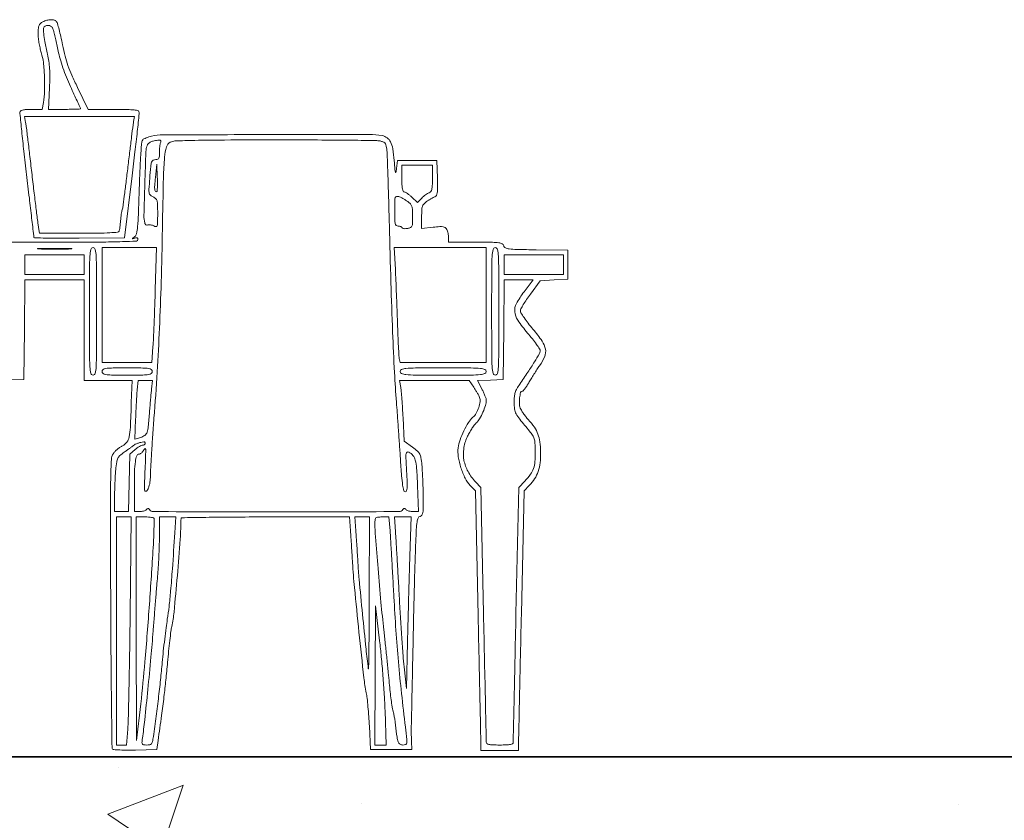
# Model space of a CAD drawing. Units: inches. Extents: x 2416 to 3391, y 1375 to 2496.
# Tile 8 of 13: x 3014 to 3044, y 2142 to 2166. Entities that reach past the tile are written whole.
import ezdxf

# ---------------------------------------------------------------- set-up
doc = ezdxf.new("R2010")
doc.units = ezdxf.units.IN
for name, color, linetype, lineweight in [('A-FLOR-PATT', 252, 'Continuous', 13), ('A-FURN', 8, 'Continuous', 18), ('A-SECT', 7, 'Continuous', 35)]:
    doc.layers.add(name, color=color, linetype=linetype, lineweight=lineweight)

msp = doc.modelspace()

# ---------------------------------------------------------------- hatches: boundary and pattern name
at = {"layer": 'A-FLOR-PATT'}
h = msp.add_hatch(dxfattribs=at)
h.set_pattern_fill('AR-CONC', color=256, scale=0.13, style=0)
h.paths.add_polyline_path([(2904.1924, 2125.8608), (3202.6924, 2125.8608), (3202.6924, 2143.8608), (2904.1924, 2143.8608)])

# ---------------------------------------------------------------- linework, layer by layer
at = {"layer": 'A-FURN'}
for points in [[(3014.6302, 2166.3653, 0.062101), (3014.5576, 2166.3165, 0.115801), (3014.5165, 2166.2593, 0.077294), (3014.4957, 2166.174, 0.016831), (3014.488, 2166.0225, 0.029474), (3014.4933, 2165.8947, 0.01481), (3014.5143, 2165.7345, 0.014652), (3014.5459, 2165.5696, 0.021013), (3014.5842, 2165.4259, -0.046916), (3014.6482, 2165.1238, -0.018058), (3014.6821, 2164.696, -0.01826), (3014.6849, 2164.2529, -0.033407), (3014.6499, 2163.8934), (3014.6158, 2163.6872), (3014.2913, 2163.6872, 0.014838), (3014.1492, 2163.683, 0.034143), (3014.0431, 2163.6694, 0.045195), (3013.9703, 2163.6479, 0.209973), (3013.9401, 2163.6175, 0.116556), (3013.9326, 2163.5615, 0.000649), (3013.9862, 2163.0221, 0.002747), (3014.0516, 2162.4062, 0.001736), (3014.1343, 2161.6884, -0.000302), (3014.219, 2160.9718, -0.000484), (3014.2903, 2160.36, -0.00008), (3014.3529, 2159.8181, -0.028704), (3014.3552, 2159.7776, 0.404392), (3014.3769, 2159.7552, 0.001815), (3014.7367, 2159.7444, 0.00627), (3015.1761, 2159.7383, 0.002975), (3015.7423, 2159.741), (3017.1294, 2159.7557), (3017.366, 2161.6502, 0.001761), (3017.4547, 2162.3815, 0.002787), (3017.5251, 2163.0091, 0.00066), (3017.5828, 2163.5587, 0.117999), (3017.5753, 2163.616, 0.260793), (3017.5322, 2163.6518, 0.023463), (3017.388, 2163.6717, 0.018121), (3017.1613, 2163.6839, 0.00441), (3016.7867, 2163.6872), (3016.0255, 2163.6872), (3015.6938, 2164.3608, -0.009259), (3015.5181, 2164.735, -0.020813), (3015.4021, 2165.0264, -0.022433), (3015.3159, 2165.3126, -0.012613), (3015.2358, 2165.6667, 0.005681), (3015.1835, 2165.914, 0.007954), (3015.1308, 2166.1335, 0.00512), (3015.0819, 2166.3158, 0.098688), (3015.0556, 2166.3678, 0.147434), (3014.9862, 2166.4165, 0.081537), (3014.8831, 2166.4329, 0.066769), (3014.7594, 2166.4155, 0.049048)], [(3014.9677, 2166.0788, -0.002772), (3014.9895, 2165.9854, -0.000537), (3015.0278, 2165.8163, -0.000571), (3015.072, 2165.619, -0.000528), (3015.117, 2165.4164, 0.019587), (3015.1803, 2165.1751, 0.01148), (3015.274, 2164.8914, 0.011132), (3015.386, 2164.5972, 0.012912), (3015.5059, 2164.3227, -0.001196), (3015.6129, 2164.0929, -0.001914), (3015.703, 2163.8961, -0.000347), (3015.7817, 2163.722, -0.1064), (3015.7849, 2163.707, -0.400461), (3015.7772, 2163.699, -0.00162), (3015.6418, 2163.693, -0.006359), (3015.4846, 2163.6886, -0.003817), (3015.2979, 2163.6872), (3014.8109, 2163.6872), (3014.8378, 2164.3414, 0.008389), (3014.8458, 2164.6704, 0.016295), (3014.8393, 2164.9332, 0.019582), (3014.8174, 2165.1589, 0.022353), (3014.7784, 2165.3724, -0.007236), (3014.6949, 2165.7627, -0.026165), (3014.6584, 2166.0142, -0.038745), (3014.6561, 2166.1759, -0.286498), (3014.699, 2166.2358, -0.083407), (3014.7937, 2166.2575, -0.147957), (3014.8708, 2166.239, -0.136318), (3014.929, 2166.1791, -0.066322)], [(3017.4133, 2163.316, 0.016785), (3017.3961, 2163.2107, 0.000753), (3017.3495, 2162.8458, 0.001264), (3017.296, 2162.4126, 0.000904), (3017.2383, 2161.9276, -0.001537), (3017.1805, 2161.4475, -0.002318), (3017.1269, 2161.0296, -0.000902), (3017.0786, 2160.6711, -0.054242), (3017.0629, 2160.608, 0.04182), (3017.0499, 2160.561, 0.008846), (3017.0357, 2160.477, 0.009204), (3017.0227, 2160.3788, 0.00862), (3017.013, 2160.278, -0.007229), (3017.0037, 2160.1783, -0.008244), (3016.9918, 2160.0831, -0.007575), (3016.9792, 2160.0028, -0.045269), (3016.9683, 2159.9619, -0.287901), (3016.9218, 2159.9259, -0.010483), (3016.6886, 2159.908, -0.011347), (3016.3351, 2159.8962, -0.002603), (3015.7378, 2159.8931), (3014.5324, 2159.8931), (3014.5, 2160.0718, -0.01368), (3014.481, 2160.1958, -0.000634), (3014.4284, 2160.618, -0.001051), (3014.3678, 2161.1195, -0.000754), (3014.3021, 2161.6802, 0.000637), (3014.2364, 2162.2409, 0.000888), (3014.1762, 2162.7424, 0.000535), (3014.1242, 2163.1647, 0.011573), (3014.106, 2163.2886), (3014.0753, 2163.4673), (3015.7593, 2163.4673), (3017.4432, 2163.4673)], [(3024.9595, 2162.7183, -0.041596), (3025.0477, 2162.6929, -0.109367), (3025.1024, 2162.657, -0.109052), (3025.1368, 2162.6013, -0.041219), (3025.16, 2162.5121, -0.033548), (3025.1735, 2162.3846, -0.000693), (3025.1969, 2161.7445, -0.00162), (3025.2208, 2160.9959, -0.001089), (3025.2435, 2160.1406, 0.001508), (3025.2916, 2158.3818, 0.00236), (3025.3448, 2156.869, 0.002712), (3025.4011, 2155.6246, 0.006937), (3025.4593, 2154.7244, -0.001348), (3025.4847, 2154.389, -0.000561), (3025.5174, 2153.9361, -0.000555), (3025.5512, 2153.4511, -0.000719), (3025.5811, 2153.0061, 0.002808), (3025.62, 2152.4624, 0.016404), (3025.6514, 2152.1773, 0.024859), (3025.6838, 2152.0105, 0.345), (3025.7291, 2151.9751, 0.316573), (3025.7694, 2152.0034, 0.06895), (3025.7879, 2152.0914, 0.02766), (3025.7902, 2152.2605, 0.003877), (3025.773, 2152.6095, -0.002437), (3025.752, 2153.011, -0.039677), (3025.7563, 2153.1458, -0.244576), (3025.7858, 2153.1897, -0.253054), (3025.8378, 2153.1899, -0.098246), (3025.9659, 2153.0848, -0.107804), (3026.039, 2152.942, -0.048185), (3026.0788, 2152.6983, -0.006257), (3026.1067, 2152.1715), (3026.1392, 2151.3702), (3025.9768, 2151.3702, -0.033091), (3025.9103, 2151.3746, -0.032649), (3025.8446, 2151.3878, -0.034456), (3025.7888, 2151.407, -0.096488), (3025.7547, 2151.43, 0.047458), (3025.7247, 2151.4547, 0.150038), (3025.7001, 2151.4623, 0.181024), (3025.6785, 2151.4542, 0.075363), (3025.6579, 2151.43, -0.259763), (3025.5466, 2151.3678, -0.00016), (3021.7784, 2151.3666, -0.00016), (3018.0103, 2151.3678, -0.259763), (3017.8989, 2151.43, 0.075363), (3017.8784, 2151.4542, 0.181024), (3017.8567, 2151.4623, 0.150038), (3017.8321, 2151.4547, 0.047458), (3017.8022, 2151.43, -0.093185), (3017.7686, 2151.407, -0.03527), (3017.7147, 2151.3878, -0.033428), (3017.6518, 2151.3746, -0.034775), (3017.5885, 2151.3702), (3017.4345, 2151.3702), (3017.4345, 2152.0782, -0.006222), (3017.4409, 2152.5964, -0.027247), (3017.4652, 2152.9016, -0.047529), (3017.5067, 2153.0799, -0.32225), (3017.5761, 2153.1298, 0.107986), (3017.6079, 2153.1367, 0.054516), (3017.6433, 2153.1579, 0.050469), (3017.6767, 2153.1889, 0.052739), (3017.7026, 2153.2256, -0.02608), (3017.7245, 2153.2604, -0.050192), (3017.7461, 2153.2853, -0.081722), (3017.7641, 2153.2973, -0.359139), (3017.7755, 2153.2943, -0.15971), (3017.7827, 2153.2713, -0.001591), (3017.78, 2153.0975, -0.004999), (3017.7742, 2152.8962, -0.003197), (3017.7637, 2152.6624, 0.004132), (3017.7535, 2152.427, 0.006129), (3017.7488, 2152.2207, 0.002969), (3017.748, 2152.0458, 0.11422), (3017.7569, 2152.008, 0.508205), (3017.8077, 2151.999, 0.112529), (3017.8653, 2152.087, 0.050052), (3017.9125, 2152.2672, 0.040546), (3017.9276, 2152.4667, -0.015334), (3017.9323, 2152.6585, -0.001578), (3017.9588, 2153.1106, -0.001966), (3017.9943, 2153.6492, -0.001569), (3018.0366, 2154.2295, 0.003613), (3018.1341, 2155.6473, 0.004281), (3018.2051, 2156.9884, 0.00402), (3018.2563, 2158.3988, 0.002606), (3018.2939, 2160.0306, -0.001427), (3018.3264, 2161.6066, -0.016729), (3018.3614, 2162.22, -0.044224), (3018.4194, 2162.5408, -0.211984), (3018.5342, 2162.6813, -0.108467), (3018.6792, 2162.7187, -0.003462), (3019.2892, 2162.7363, -0.004434), (3020.1924, 2162.7481, -0.000997), (3021.7303, 2162.7516, -0.001043), (3022.9149, 2162.7495, -0.001602), (3023.9406, 2162.7422, -0.000518), (3024.8287, 2162.7321, -0.046286)], [(3018.2377, 2162.6655, 0.050508), (3018.2248, 2162.618, 0.013659), (3018.2141, 2162.5407, 0.013682), (3018.2068, 2162.4519, 0.013799), (3018.2043, 2162.363, -0.018316), (3018.2001, 2162.2491, -0.096973), (3018.1837, 2162.1891, -0.179316), (3018.1513, 2162.1585, -0.100622), (3018.0976, 2162.1476, 0.12004), (3018.0115, 2162.1266, 0.195826), (3017.9634, 2162.0702, 0.057245), (3017.9368, 2161.9425, 0.003765), (3017.9055, 2161.5668, 0.004039), (3017.8833, 2161.238, 0.060235), (3017.8902, 2161.1233, 0.16542), (3017.9266, 2161.0582, 0.076736), (3018.0085, 2161.0044, -0.076881), (3018.0886, 2160.9518, -0.142342), (3018.1292, 2160.8861, -0.061734), (3018.146, 2160.7732, -0.00604), (3018.1493, 2160.4972, -0.003502), (3018.1473, 2160.2093, -0.069301), (3018.1339, 2160.1221, -0.344095), (3018.0994, 2160.0977, -0.111915), (3018.035, 2160.1154, 0.041765), (3017.9858, 2160.1367, 0.038588), (3017.9324, 2160.1501, 0.040889), (3017.8828, 2160.1545, 0.093547), (3017.846, 2160.1479, -0.120448), (3017.8157, 2160.144, -0.121496), (3017.7871, 2160.1546, -0.108755), (3017.7645, 2160.1785, -0.081976), (3017.7511, 2160.2124, -0.059517), (3017.7298, 2160.4363, -0.001663), (3017.7566, 2161.4086, -0.001289), (3017.7896, 2162.3985, -0.080665), (3017.8238, 2162.5695, -0.101839), (3017.8673, 2162.6388, -0.091995), (3017.9361, 2162.6883, -0.062829), (3018.0405, 2162.7223, -0.02224), (3018.1964, 2162.7449, -0.10297), (3018.225, 2162.7419, -0.197977), (3018.2423, 2162.7273, -0.154104), (3018.2468, 2162.7014, -0.058414)], [(3018.1244, 2161.1695, -0.395847), (3018.0853, 2161.1683, -0.188529), (3018.0602, 2161.217, -0.04324), (3018.0579, 2161.3556, -0.008525), (3018.0795, 2161.6034), (3018.1218, 2162.0101), (3018.1381, 2161.6048, -0.007181), (3018.1422, 2161.4474, -0.010754), (3018.1408, 2161.3098, -0.005966), (3018.1358, 2161.1951, -0.184544)], [(3026.5623, 2161.5739, -0.007704), (3026.5588, 2161.3473, -0.048789), (3026.544, 2161.233, -0.111409), (3026.5134, 2161.1693, -0.14956), (3026.461, 2161.1331, 0.058669), (3026.4134, 2161.1116, 0.022268), (3026.3527, 2161.0713, 0.021691), (3026.2899, 2161.0211, 0.024771), (3026.2345, 2160.9677), (3026.1094, 2160.8345), (3025.9372, 2160.9959, 0.018241), (3025.8662, 2161.0577, 0.022282), (3025.7953, 2161.11, 0.021517), (3025.733, 2161.148, 0.125972), (3025.6962, 2161.1576, -0.306893), (3025.6642, 2161.1794, -0.052792), (3025.6435, 2161.254, -0.032091), (3025.631, 2161.3776, -0.009182), (3025.6275, 2161.5702), (3025.6275, 2161.9826), (3026.0949, 2161.9826), (3026.5623, 2161.9826)], [(3025.8051, 2160.8648, -0.04726), (3025.8894, 2160.7893, -0.105675), (3025.933, 2160.7156, -0.06907), (3025.9526, 2160.6116, -0.012071), (3025.9574, 2160.4116, -0.007911), (3025.954, 2160.1971, -0.089309), (3025.9364, 2160.1142, -0.189388), (3025.8942, 2160.07, -0.06065), (3025.8062, 2160.0415, -0.032494), (3025.7469, 2160.034, -0.04645), (3025.694, 2160.0356, -0.05614), (3025.6541, 2160.0452, -0.222131), (3025.6367, 2160.0626, 0.149945), (3025.6221, 2160.082, 0.060016), (3025.5927, 2160.0983, 0.052195), (3025.5546, 2160.1093, 0.044695), (3025.5129, 2160.1131, -0.18104), (3025.4566, 2160.1342, -0.159918), (3025.4244, 2160.1883, -0.050048), (3025.4103, 2160.3044, -0.005016), (3025.4075, 2160.5842, -0.003519), (3025.4097, 2160.8921, -0.065713), (3025.4237, 2160.9879, -0.288466), (3025.4606, 2161.0211, -0.120126), (3025.5302, 2161.0163, -0.034306), (3025.5879, 2160.9935, -0.014795), (3025.6616, 2160.9558, -0.014559), (3025.7378, 2160.9108, -0.018684)], [(3015.4714, 2159.4124, -0.006561), (3015.2639, 2159.4066, -0.003649), (3015.0108, 2159.4047, -0.003639), (3014.7546, 2159.4066, -0.005878), (3014.5366, 2159.4123, -0.030672), (3014.4692, 2159.419, -0.903981), (3014.4695, 2159.4253, -0.008594), (3014.6526, 2159.4296, -0.001615), (3014.9876, 2159.4307, -0.001661), (3015.3231, 2159.4297, -0.007856), (3015.5153, 2159.4254, -0.862966), (3015.516, 2159.419, -0.053751)], [(3016.2798, 2157.5012, -0.000789), (3016.2778, 2156.2278, -0.013281), (3016.2653, 2155.8069, -0.040964), (3016.2369, 2155.6029, -0.351139), (3016.1698, 2155.5492, -0.351139), (3016.1027, 2155.6029, -0.040964), (3016.0743, 2155.8069, -0.013281), (3016.0618, 2156.2278, -0.000789), (3016.0598, 2157.5012, -0.000789), (3016.0618, 2158.7746, -0.013281), (3016.0743, 2159.1955, -0.040964), (3016.1027, 2159.3995, -0.351139), (3016.1698, 2159.4532, -0.351139), (3016.2369, 2159.3995, -0.040964), (3016.2653, 2159.1955, -0.013281), (3016.2778, 2158.7746, -0.000789)], [(3018.0752, 2158.1748, -0.001517), (3018.0589, 2157.6501, -0.001562), (3018.0395, 2157.1306, -0.001509), (3018.0199, 2156.6803, -0.006657), (3018.0041, 2156.4152), (3017.9689, 2155.9341), (3017.2068, 2155.9341), (3016.4447, 2155.9341), (3016.4447, 2157.6937), (3016.4447, 2159.4532), (3017.2779, 2159.4532), (3018.1111, 2159.4532)], [(3028.2119, 2157.6937), (3028.2119, 2155.9341), (3026.8932, 2155.9341), (3025.5746, 2155.9341), (3025.5495, 2156.0578, -0.035598), (3025.5384, 2156.1435, -0.001758), (3025.5229, 2156.4279, -0.002835), (3025.5076, 2156.7662, -0.002044), (3025.4942, 2157.1438, 0.001348), (3025.4799, 2157.5615, 0.001011), (3025.4621, 2158.0213, 0.001022), (3025.4435, 2158.4539, 0.002346), (3025.4274, 2158.7797), (3025.3908, 2159.4532), (3026.8013, 2159.4532), (3028.2119, 2159.4532)], [(3028.5968, 2157.5012, -0.000789), (3028.5948, 2156.2278, -0.013281), (3028.5822, 2155.8069, -0.040964), (3028.5539, 2155.6029, -0.351139), (3028.4868, 2155.5492, -0.351139), (3028.4197, 2155.6029, -0.040964), (3028.3913, 2155.8069, -0.013281), (3028.3788, 2156.2278, -0.000789), (3028.3768, 2157.5012, -0.000789), (3028.3788, 2158.7746, -0.013281), (3028.3913, 2159.1955, -0.040964), (3028.4197, 2159.3995, -0.351139), (3028.4868, 2159.4532, -0.351139), (3028.5539, 2159.3995, -0.040964), (3028.5822, 2159.1955, -0.013281), (3028.5948, 2158.7746, -0.000789)], [(3029.3684, 2158.0979, 0.036037), (3029.1362, 2157.7403, 0.148447), (3029.0832, 2157.4906, 0.129492), (3029.1748, 2157.2343, 0.024803), (3029.4765, 2156.8376, -0.008208), (3029.624, 2156.6566, -0.011718), (3029.7484, 2156.4908, -0.007772), (3029.8461, 2156.3494, -0.148348), (3029.8615, 2156.2987, -0.130297), (3029.8376, 2156.2086, -0.007082), (3029.6871, 2155.9532, -0.010099), (3029.4883, 2155.6408, -0.005901), (3029.2382, 2155.2743, 0.023411), (3029.1482, 2155.132, 0.053399), (3029.0976, 2155.0156, 0.052936), (3029.0725, 2154.8906, 0.022659), (3029.0646, 2154.7201, 0.034382), (3029.0789, 2154.5083, 0.08877), (3029.1259, 2154.3631, 0.048451), (3029.2357, 2154.1981, 0.004972), (3029.5356, 2153.8375, -0.031451), (3029.6314, 2153.7091, -0.076691), (3029.6799, 2153.6019, -0.05417), (3029.7027, 2153.464, -0.009879), (3029.7119, 2153.2051, -0.021459), (3029.7034, 2152.8923, -0.068458), (3029.6606, 2152.6883, -0.075136), (3029.5668, 2152.5138, -0.029552), (3029.39, 2152.305), (3029.2066, 2152.1125), (3029.1216, 2148.2468, 0.000042), (3029.089, 2146.7591, 0.000068), (3029.0616, 2145.4933, 0.000009), (3029.0373, 2144.3653, 0.005374), (3029.0367, 2144.3015, -0.262499), (3029.0147, 2144.2626, -0.088563), (3028.9517, 2144.2384, -0.039752), (3028.8347, 2144.2253, -0.007928), (3028.6243, 2144.222, -0.00722), (3028.4026, 2144.2252, -0.045238), (3028.2902, 2144.2386, -0.11622), (3028.2331, 2144.2656, -0.228425), (3028.2119, 2144.3097, 0.005402), (3028.2111, 2144.3798, 0.000011), (3028.1868, 2145.5049, 0.000076), (3028.1592, 2146.7698, 0.000047), (3028.1264, 2148.255), (3028.041, 2152.1125), (3027.8851, 2152.2775, -0.063024), (3027.6532, 2152.5949, -0.079397), (3027.5297, 2152.9366, -0.081985), (3027.5209, 2153.2911, -0.072747), (3027.6244, 2153.6455, -0.018882), (3027.6887, 2153.7731, -0.016494), (3027.7653, 2153.9015, -0.016801), (3027.8423, 2154.013, -0.046374), (3027.906, 2154.084, 0.072272), (3028.009, 2154.2117, 0.029932), (3028.1107, 2154.4095, 0.029898), (3028.188, 2154.6176, 0.074023), (3028.2119, 2154.7781, 0.077201), (3028.2038, 2154.8301, 0.015225), (3028.1723, 2154.9195, 0.015805), (3028.1287, 2155.0223, 0.014097), (3028.0772, 2155.1263), (3027.9425, 2155.3795), (3028.3384, 2155.3956), (3028.7342, 2155.4117), (3028.7488, 2156.9376), (3028.7635, 2158.4635), (3029.2043, 2158.4635), (3029.6452, 2158.4635)], [(3017.9844, 2155.6592, -0.235138), (3017.9539, 2155.598, -0.126958), (3017.8744, 2155.5649, -0.033055), (3017.6985, 2155.5515, -0.002431), (3017.2145, 2155.5492, -0.002431), (3016.7306, 2155.5515, -0.033055), (3016.5547, 2155.5649, -0.126958), (3016.4752, 2155.598, -0.235138), (3016.4447, 2155.6592, -0.235138), (3016.4752, 2155.7203, -0.126958), (3016.5547, 2155.7534, -0.033055), (3016.7306, 2155.7668, -0.002431), (3017.2145, 2155.7691, -0.002431), (3017.6985, 2155.7668, -0.033055), (3017.8744, 2155.7534, -0.126958), (3017.9539, 2155.7203, -0.235138)], [(3028.2119, 2155.6592, -0.309944), (3028.1679, 2155.595, -0.07148), (3028.0331, 2155.5641, -0.019546), (3027.7433, 2155.5513, -0.001241), (3026.8922, 2155.5492, -0.001241), (3026.0411, 2155.5513, -0.019546), (3025.7512, 2155.5641, -0.07148), (3025.6165, 2155.595, -0.309944), (3025.5725, 2155.6592, -0.309944), (3025.6165, 2155.7233, -0.07148), (3025.7512, 2155.7542, -0.019546), (3026.0411, 2155.767, -0.001241), (3026.8922, 2155.7691, -0.001241), (3027.7433, 2155.767, -0.019546), (3028.0331, 2155.7542, -0.07148), (3028.1679, 2155.7233, -0.309944)], [(3017.9634, 2155.123, 0.005266), (3017.9492, 2154.9926, 0.001969), (3017.9319, 2154.8094, 0.001951), (3017.9146, 2154.6095, 0.002364), (3017.9, 2154.422, -0.005337), (3017.8625, 2153.975, -0.058462), (3017.8248, 2153.7991, -0.147783), (3017.7573, 2153.7048, -0.089797), (3017.6344, 2153.6413), (3017.4544, 2153.5861), (3017.4735, 2154.1965, -0.003004), (3017.483, 2154.4513, -0.002792), (3017.4958, 2154.7124, -0.002783), (3017.5097, 2154.9444, -0.009418), (3017.5225, 2155.0956), (3017.5524, 2155.3842), (3017.7735, 2155.3842), (3017.9947, 2155.3842)], [(3017.7644, 2153.4597, -0.133438), (3017.7587, 2153.4387, -0.100502), (3017.7427, 2153.4209, -0.08749), (3017.7187, 2153.4089, -0.072739), (3017.6905, 2153.4047, 0.109307), (3017.6519, 2153.3962, 0.023905), (3017.5913, 2153.3644, 0.023809), (3017.5234, 2153.32, 0.020876), (3017.4568, 2153.2674), (3017.297, 2153.1302), (3017.2775, 2152.2502), (3017.258, 2151.3702), (3017.0438, 2151.3702), (3016.8296, 2151.3702), (3016.83, 2151.8239, -0.006353), (3016.8328, 2152.025, -0.004256), (3016.8408, 2152.255, -0.004286), (3016.8523, 2152.4777, -0.008427), (3016.866, 2152.6545, -0.011499), (3016.8937, 2152.8898, -0.078491), (3016.9278, 2153.0012, -0.101428), (3016.9914, 2153.0839, -0.025172), (3017.1268, 2153.1896, 0.002136), (3017.2175, 2153.2539, 0.00244), (3017.3036, 2153.3161, 0.002205), (3017.3762, 2153.3696, 0.01383), (3017.4124, 2153.3981, -0.063042), (3017.4635, 2153.4308, -0.025549), (3017.54, 2153.4624, -0.023998), (3017.6298, 2153.4895, -0.02284), (3017.7232, 2153.5083, -0.137055), (3017.7389, 2153.5064, -0.119526), (3017.7523, 2153.4967, -0.101269), (3017.7613, 2153.4802, -0.07511)], [(3017.3058, 2148.1947, -0.000924), (3017.2897, 2147.0066, -0.001232), (3017.2704, 2145.9272, -0.000862), (3017.2504, 2145.0221, -0.012597), (3017.2348, 2144.7031), (3017.199, 2144.222), (3017.0418, 2144.222), (3016.8846, 2144.222), (3016.8846, 2147.7136), (3016.8846, 2151.2053), (3017.1129, 2151.2053), (3017.3411, 2151.2053)], [(3018.0393, 2151.1583, -0.015434), (3018.0117, 2150.2643, -0.002533), (3017.8963, 2148.5382, -0.002966), (3017.7581, 2146.7652, -0.00764), (3017.6311, 2145.4867), (3017.5017, 2144.3594), (3017.4956, 2147.7823), (3017.4895, 2151.2053), (3017.7644, 2151.2053, -0.016049), (3017.8698, 2151.2019, -0.02622), (3017.9586, 2151.1915, -0.024296), (3018.0253, 2151.1767, -0.338224)], [(3018.6756, 2150.7241, -0.00103), (3018.5999, 2149.6151, -0.004128), (3018.5466, 2148.9371, -0.006674), (3018.4987, 2148.4609, -0.011909), (3018.4449, 2148.071, 0.007646), (3018.4073, 2147.8152, 0.003159), (3018.364, 2147.4679, 0.003124), (3018.3222, 2147.0948, 0.004017), (3018.2886, 2146.7513, -0.004388), (3018.2366, 2146.222, -0.003277), (3018.1702, 2145.6394, -0.003125), (3018.0923, 2145.0252, -0.002957), (3018.0053, 2144.4007, -0.029706), (3017.985, 2144.3022, -0.13851), (3017.9556, 2144.253, -0.15221), (3017.9064, 2144.2289, -0.038268), (3017.8163, 2144.222, -0.027758), (3017.7175, 2144.2275, -0.224413), (3017.6799, 2144.2506, -0.166457), (3017.6677, 2144.299, -0.014147), (3017.6821, 2144.4282, 0.008037), (3017.752, 2144.9907, 0.001948), (3017.8488, 2145.9227, 0.002109), (3017.9432, 2146.9084, 0.003771), (3018.0112, 2147.7195, -0.000707), (3018.047, 2148.1806, -0.000623), (3018.0857, 2148.6616, -0.000625), (3018.1216, 2149.0954, -0.001891), (3018.1476, 2149.3907, 0.007329), (3018.1681, 2149.6564, 0.004095), (3018.1856, 2149.9802, 0.004084), (3018.1979, 2150.3079, 0.006623), (3018.2024, 2150.5867), (3018.2043, 2151.2053), (3018.4559, 2151.2053), (3018.7074, 2151.2053)], [(3024.6295, 2148.7996, -0.000858), (3024.6248, 2147.8882, -0.001595), (3024.6174, 2147.1491, -0.000779), (3024.6087, 2146.5594, -0.929775), (3024.5998, 2146.5589, -0.006494), (3024.5295, 2147.1615, -0.001321), (3024.4217, 2148.2308, -0.001169), (3024.3191, 2149.3007, -0.008991), (3024.2813, 2149.8031, 0.001088), (3024.2669, 2150.0447, 0.000764), (3024.2497, 2150.3166, 0.000771), (3024.2324, 2150.5768, 0.001616), (3024.2181, 2150.7791), (3024.1864, 2151.2053), (3024.4121, 2151.2053), (3024.6377, 2151.2053)], [(3025.2646, 2150.7791, -0.004324), (3025.2823, 2150.5253, -0.000632), (3025.3132, 2150.0097, -0.000714), (3025.348, 2149.4001, -0.000612), (3025.383, 2148.7584, 0.004039), (3025.4458, 2147.7348, 0.004765), (3025.5223, 2146.7674, 0.004749), (3025.6175, 2145.7988, 0.003962), (3025.7365, 2144.7718, -0.002622), (3025.7816, 2144.3919, -0.06314), (3025.7802, 2144.2851, -0.266706), (3025.7441, 2144.2386, -0.097511), (3025.6593, 2144.222, -0.140768), (3025.5709, 2144.2474, -0.16522), (3025.5161, 2144.3146, -0.055683), (3025.4795, 2144.4611, -0.005325), (3025.4341, 2144.8268, 0.008409), (3025.4175, 2144.9547, 0.007185), (3025.3958, 2145.0889, 0.007254), (3025.3725, 2145.2103, 0.020393), (3025.3515, 2145.2942, -0.033712), (3025.3293, 2145.3944, -0.004728), (3025.2994, 2145.6045, -0.005383), (3025.269, 2145.8543, -0.004551), (3025.2421, 2146.119, 0.001908), (3025.2113, 2146.4393, 0.000813), (3025.1677, 2146.8677, 0.000805), (3025.1197, 2147.3244, 0.001058), (3025.0744, 2147.7411, -0.004372), (3024.9876, 2148.5914, -0.002477), (3024.8965, 2149.6227, -0.001751), (3024.8186, 2150.5999, -0.018582), (3024.8031, 2150.9991, -0.018903), (3024.8077, 2151.1293, -0.1845), (3024.8307, 2151.1783, -0.176568), (3024.8811, 2151.2006, -0.017026), (3025.0169, 2151.2053), (3025.2311, 2151.2053)], [(3025.8717, 2150.0093, 0.000601), (3025.8549, 2149.4491, 0.000306), (3025.8351, 2148.7447, 0.000304), (3025.8155, 2148.0182, 0.000455), (3025.7994, 2147.3837), (3025.7643, 2145.954), (3025.6954, 2146.6139, -0.006964), (3025.6635, 2146.9656, -0.00188), (3025.6229, 2147.5241, -0.001903), (3025.5817, 2148.1585, -0.001971), (3025.5457, 2148.7858, 0.000567), (3025.5124, 2149.398, 0.000636), (3025.4789, 2149.987, 0.000583), (3025.4491, 2150.4884, 0.003423), (3025.4314, 2150.7516), (3025.3977, 2151.2053), (3025.6533, 2151.2053), (3025.909, 2151.2053)], [(3025.1117, 2145.2805), (3025.1493, 2144.222), (3024.976, 2144.222), (3024.8027, 2144.222), (3024.8098, 2146.3527), (3024.8169, 2148.4834), (3024.9455, 2147.4112, -0.006504), (3024.9975, 2146.924, -0.003877), (3025.0474, 2146.343, -0.00388), (3025.0881, 2145.7632, -0.006704)]]:
    msp.add_lwpolyline(points, format="xyb", close=True, dxfattribs=at)
msp.add_lwpolyline([(3012.8543, 2155.3969), (3014.0528, 2155.4117), (3014.0674, 2156.9376), (3014.082, 2158.4635), (3014.9885, 2158.4635), (3015.8949, 2158.4635), (3015.8949, 2156.9239), (3015.8949, 2155.3842), (3016.6293, 2155.3842), (3017.3638, 2155.3842), (3017.3424, 2154.7107, -0.003328), (3017.3131, 2153.9508, -0.038266), (3017.2769, 2153.6542, -0.110047), (3017.2063, 2153.4949, -0.122943), (3017.0769, 2153.3882, 0.037278), (3016.9982, 2153.3432, 0.025768), (3016.9162, 2153.2814, 0.026073), (3016.8431, 2153.2135, 0.047392), (3016.7922, 2153.1499, 0.133252), (3016.7314, 2152.9632, 0.008115), (3016.7113, 2152.3711, 0.004957), (3016.7031, 2151.315, 0.000411), (3016.7112, 2148.5701, 0.000878), (3016.7206, 2146.8682, 0.001443), (3016.7352, 2145.4283, 0.000121), (3016.7524, 2144.1381, 0.191181), (3016.7696, 2144.0964, 0.187976), (3016.8062, 2144.0797, 0.004747), (3016.9915, 2144.0706, 0.009523), (3017.2124, 2144.0661, 0.006273), (3017.4666, 2144.0689), (3018.1218, 2144.0845), (3018.1611, 2144.3594, 0.0016), (3018.2682, 2145.1259, 0.003707), (3018.3425, 2145.7019, 0.004453), (3018.3996, 2146.2098, 0.003691), (3018.4515, 2146.7513, -0.003413), (3018.4844, 2147.0958, -0.003857), (3018.5207, 2147.426, -0.003526), (3018.5557, 2147.7061, -0.021069), (3018.5812, 2147.8511, 0.029976), (3018.6504, 2148.292, 0.002672), (3018.7519, 2149.4105, 0.003466), (3018.839, 2150.523, 0.01627), (3018.8639, 2151.164, -0.407437), (3018.8806, 2151.1809, -0.000252), (3019.6215, 2151.1931, -0.002499), (3020.454, 2151.2023, -0.001499), (3021.4428, 2151.2053), (3024.0214, 2151.2053), (3024.0531, 2150.7791, -0.001613), (3024.0675, 2150.5768, -0.000769), (3024.0847, 2150.3166, -0.000763), (3024.1019, 2150.0447, -0.001085), (3024.1163, 2149.8031, 0.010025), (3024.1752, 2149.0434, 0.001946), (3024.3143, 2147.6748, 0.001328), (3024.4651, 2146.2813, 0.021641), (3024.5371, 2145.8166, -0.020675), (3024.5626, 2145.6541, -0.005491), (3024.5897, 2145.393, -0.005559), (3024.614, 2145.0952, -0.005699), (3024.6314, 2144.7993), (3024.6652, 2144.0845), (3025.2976, 2144.0845), (3025.9299, 2144.0845), (3025.9206, 2144.3319, -0.014355), (3025.9168, 2144.7727, -0.000291), (3025.9625, 2146.9939, -0.000702), (3026.0098, 2149.0939, -0.003447), (3026.0464, 2150.2796, -0.002482), (3026.0698, 2150.8254, -0.024335), (3026.0919, 2151.0548, -0.066388), (3026.1255, 2151.1728, -0.230155), (3026.1842, 2151.223, 0.186381), (3026.2397, 2151.263, 0.106397), (3026.2697, 2151.3413, 0.03719), (3026.2819, 2151.4933, 0.004012), (3026.2809, 2151.8462, 0.004454), (3026.2759, 2152.1006, 0.003663), (3026.2661, 2152.3721, 0.003699), (3026.2535, 2152.6214, 0.009807), (3026.2397, 2152.7992, 0.013851), (3026.2116, 2153.0225, 0.083765), (3026.1751, 2153.1328, 0.093053), (3026.1058, 2153.2198, 0.019095), (3025.9517, 2153.343), (3025.6986, 2153.53), (3025.6624, 2154.2451, 0.002929), (3025.6461, 2154.5344, 0.003294), (3025.6269, 2154.8124, 0.003021), (3025.6076, 2155.0487, 0.017756), (3025.5923, 2155.1722), (3025.5584, 2155.3842), (3026.624, 2155.3836), (3027.6895, 2155.3829), (3027.8269, 2155.1774, -0.008157), (3027.8827, 2155.091, -0.007763), (3027.9366, 2155.0014, -0.007733), (3027.9817, 2154.9208, -0.027137), (3028.0071, 2154.867, -0.128906), (3028.0241, 2154.7366, -0.050122), (3027.9829, 2154.5579, -0.049339), (3027.9033, 2154.382, -0.08259), (3027.8004, 2154.257, 0.074138), (3027.6662, 2154.0995, 0.027382), (3027.5253, 2153.8432, 0.027659), (3027.4091, 2153.5628, 0.05034), (3027.351, 2153.322, 0.075633), (3027.355, 2153.0513, 0.036071), (3027.4372, 2152.7121, 0.036071), (3027.5673, 2152.3885, 0.076326), (3027.7209, 2152.167), (3027.8779, 2152.0015), (3027.9622, 2148.1805, -0.000078), (3027.9946, 2146.7049, -0.000122), (3028.0218, 2145.4374, -0.000028), (3028.0454, 2144.326, -0.005012), (3028.0467, 2144.2082), (3028.0469, 2144.057), (3028.6243, 2144.057), (3029.2016, 2144.057), (3029.2018, 2144.2632, -0.005063), (3029.2035, 2144.4203, -0.000053), (3029.2265, 2145.515, -0.00017), (3029.2537, 2146.7769, -0.00011), (3029.2859, 2148.2351), (3029.37, 2152.0008), (3029.5304, 2152.1666, 0.051232), (3029.6935, 2152.3739, 0.059972), (3029.801, 2152.5997, 0.053601), (3029.8597, 2152.8649, 0.03075), (3029.8757, 2153.1925, 0.027873), (3029.8542, 2153.5067, 0.060337), (3029.7957, 2153.7412, 0.061521), (3029.6838, 2153.9521, 0.030014), (3029.4941, 2154.1912, -0.016925), (3029.4184, 2154.2816, -0.0151), (3029.3459, 2154.3803, -0.015334), (3029.2862, 2154.4731, -0.044549), (3029.2529, 2154.5416, -0.082824), (3029.2259, 2154.6764, -0.038521), (3029.2338, 2154.855, -0.034312), (3029.2646, 2155.0152, -0.340396), (3029.3154, 2155.0543, 0.220282), (3029.3405, 2155.0659, 0.013892), (3029.3927, 2155.131, 0.018365), (3029.4518, 2155.2154, 0.012463), (3029.5131, 2155.3155, -0.006759), (3029.584, 2155.4343, -0.003819), (3029.6731, 2155.5765, -0.003812), (3029.765, 2155.7186, -0.006248), (3029.8453, 2155.8373, 0.05273), (3030.0009, 2156.1207, 0.145222), (3030.0252, 2156.345, 0.107892), (3029.9241, 2156.5872, 0.022406), (3029.6415, 2156.9551, -0.010359), (3029.4941, 2157.1377, -0.014209), (3029.3697, 2157.3084, -0.010889), (3029.2743, 2157.4539, -0.140429), (3029.2566, 2157.5158, -0.122754), (3029.2718, 2157.5768, -0.012236), (3029.3462, 2157.7089, -0.014813), (3029.4449, 2157.8637, -0.011247), (3029.5617, 2158.0277), (3029.8668, 2158.436), (3030.2903, 2158.4635), (3030.7137, 2158.491), (3030.7137, 2158.9309), (3030.7137, 2159.3708), (3029.7438, 2159.3858, -0.002065), (3029.1428, 2159.3975, -0.024901), (3028.9122, 2159.4145, -0.077982), (3028.7973, 2159.4474, -0.223731), (3028.7455, 2159.5095, 0.207405), (3028.6977, 2159.5704, 0.093017), (3028.5989, 2159.6022, 0.029057), (3028.4004, 2159.6157, 0.002451), (3027.8871, 2159.6182), (3027.0571, 2159.6182), (3027.0571, 2159.7593, 0.033836), (3027.0529, 2159.8212, 0.023076), (3027.0402, 2159.8905, 0.023315), (3027.0216, 2159.9566, 0.04267), (3026.9995, 2160.008, 0.098776), (3026.9532, 2160.0643, 0.129324), (3026.8929, 2160.0918, 0.06006), (3026.7935, 2160.0969, 0.00832), (3026.5871, 2160.0793), (3026.2323, 2160.0429), (3026.2323, 2160.3976, -0.011031), (3026.237, 2160.6074, -0.067682), (3026.2562, 2160.7136, -0.107955), (3026.2995, 2160.7876, -0.049059), (3026.3836, 2160.8625, -0.013143), (3026.4486, 2160.9074, -0.011369), (3026.5192, 2160.9511, -0.011512), (3026.585, 2160.9878, -0.032422), (3026.633, 2161.0094, 0.172342), (3026.6846, 2161.0526, 0.097543), (3026.7119, 2161.1306, 0.038158), (3026.7215, 2161.2741, 0.00489), (3026.7155, 2161.583), (3026.6997, 2162.1201), (3026.0949, 2162.1201), (3025.49, 2162.1201), (3025.4617, 2161.8726, -0.01645), (3025.4447, 2161.758, -0.793795), (3025.4309, 2161.7574, -0.046655), (3025.4168, 2161.8332, -0.0018), (3025.3917, 2162.1178, 0.018072), (3025.3478, 2162.4807, 0.074304), (3025.2816, 2162.6914, 0.126004), (3025.1772, 2162.8143, 0.105108), (3025.0195, 2162.8823, 0.049609), (3024.6338, 2162.9203, 0.00038), (3021.4796, 2162.9151, 0.000338), (3018.3077, 2162.9054, 0.056116), (3017.9639, 2162.8654, 0.018566), (3017.878, 2162.842, 0.019793), (3017.7959, 2162.8128, 0.019817), (3017.7276, 2162.7823, 0.081365), (3017.6909, 2162.7559, 0.17725), (3017.6626, 2162.6949, 0.003341), (3017.6351, 2162.3388, 0.006837), (3017.6093, 2161.8838, 0.003004), (3017.587, 2161.2807, -0.00174), (3017.559, 2160.4682, -0.013822), (3017.5344, 2160.0932, -0.026664), (3017.5029, 2159.8799, -0.176367), (3017.4476, 2159.7895, 0.001975), (3017.3841, 2159.7385, 0.230336), (3017.3797, 2159.7291, 0.505939), (3017.3851, 2159.7253, 0.003457), (3017.4482, 2159.7465, -0.054737), (3017.4896, 2159.7559, -0.139774), (3017.5197, 2159.7509, -0.180631), (3017.5379, 2159.7322, -0.103785), (3017.5445, 2159.701, -0.398581), (3017.4999, 2159.654, -0.005599), (3017.0742, 2159.6359, -0.006647), (3016.3856, 2159.6235, -0.000887), (3014.9326, 2159.6193), (3012.3207, 2159.6163)], format="xyb", dxfattribs=at)
for points in [[(3015.8949, 2158.9309), (3015.8949, 2158.6284), (3014.9876, 2158.6284), (3014.0803, 2158.6284), (3014.0803, 2158.9309), (3014.0803, 2159.2333), (3014.9876, 2159.2333), (3015.8949, 2159.2333)], [(3030.5763, 2158.9309), (3030.5763, 2158.6284), (3029.669, 2158.6284), (3028.7617, 2158.6284), (3028.7617, 2158.9309), (3028.7617, 2159.2333), (3029.669, 2159.2333), (3030.5763, 2159.2333)]]:
    msp.add_lwpolyline(points, close=True, dxfattribs=at)
at = {"layer": 'A-SECT'}
msp.add_line((3202.6924, 2143.8608), (2904.1924, 2143.8608), dxfattribs=at)

doc.saveas('drawing.dxf')
